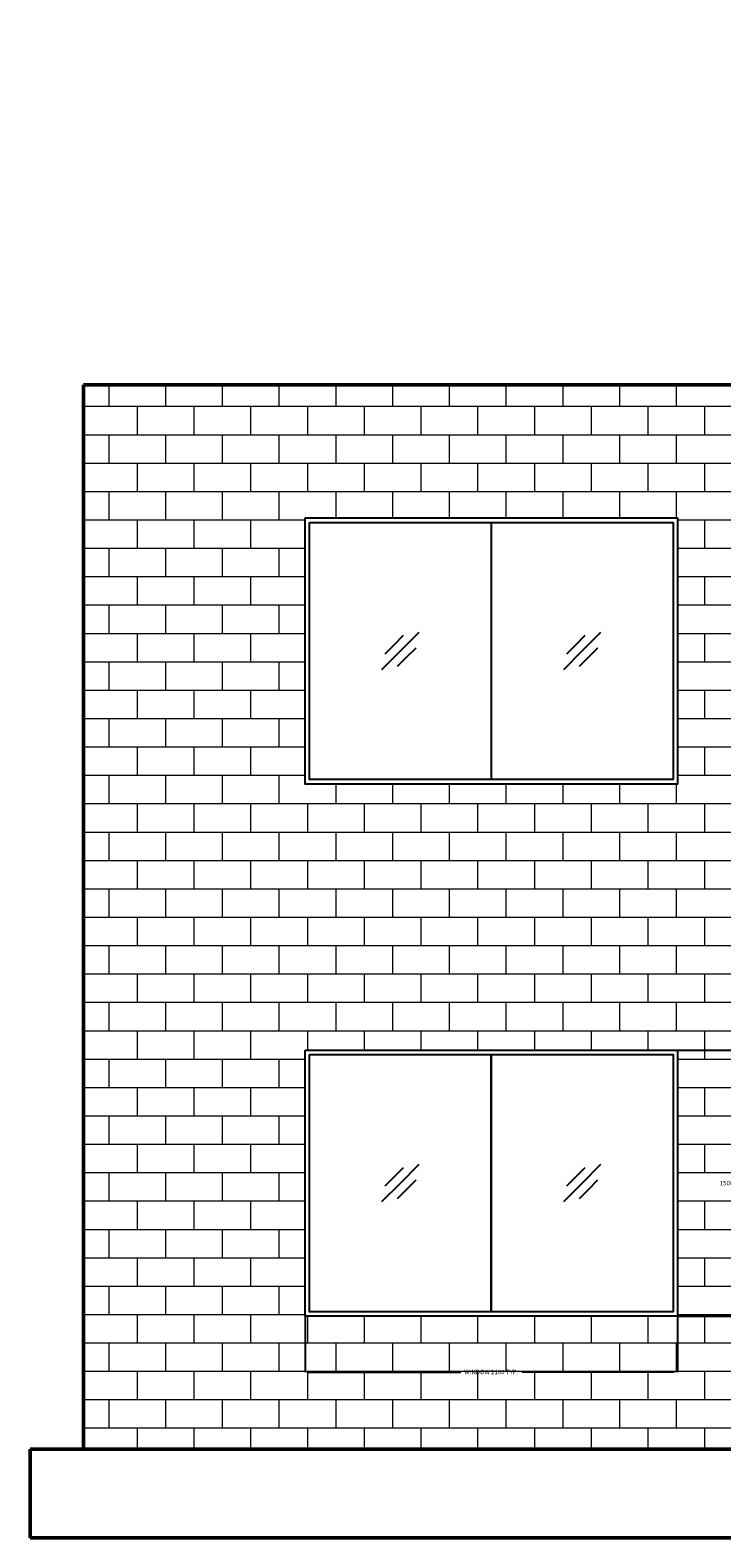
# Model space of a CAD drawing. Units: centimetres. Extents: x 2755 to 12755, y 4821 to 13321.
# Tile 1 of 2: x 2755 to 6655, y 4821 to 13321. Entities that reach past the tile are written whole.
import ezdxf

# ---------------------------------------------------------------- set-up
doc = ezdxf.new("R2010")
doc.units = ezdxf.units.CM
doc.header["$MEASUREMENT"] = 0
for name, color, linetype, lineweight in [('A-ANNO-DIMS', 2, 'Continuous', 18), ('A-GLAZ', 4, 'Continuous', 25), ('A-WALL', 7, 'Continuous', 50), ('A-WALL-PATT', 8, 'Continuous', 13)]:
    doc.layers.add(name, color=color, linetype=linetype, lineweight=lineweight)
doc.styles.get("Standard").update_dxf_attribs({"font": 'arial.ttf'})
doc.dimstyles.get("Standard").update_dxf_attribs({"dimtxt": 25, "dimasz": 20, "dimexe": 0.18, "dimexo": 0.0625, "dimgap": 10, "dimtad": 0, "dimtih": 1, "dimtoh": 1, "dimdec": 0, "dimzin": 0, "dimdsep": 46, "dimtxsty": 'Standard', "dimcen": 10, "dimadec": 0, "dimazin": 0, "dimtfac": 1, "dimtdec": 0, "dimtofl": 0, "dimtmove": 0, "dimatfit": 3, "dimfxl": 1, "dimtolj": 1, "dimtzin": 0, "dimarcsym": 0})

# ---------------------------------------------------------------- blocks, each defined once
blk = doc.blocks.new('WIN-2100')
blk.add_line((5355.3, 7545.8), (5355.3, 6095.8))
for points in [[(4305.3, 7570.8), (6405.3, 7570.8), (6405.3, 6070.8), (4305.3, 6070.8)], [(4330.3, 7545.8), (6380.3, 7545.8), (6380.3, 6095.8), (4330.3, 6095.8)]]:
    blk.add_lwpolyline(points, close=True)
blk = doc.blocks.new('*D4')
at = {"layer": 'A-ANNO-DIMS', "color": 0, "lineweight": -2, "transparency": 16777216}
for p, q in [((4305.3, 6070.8), (4305.3, 5755.6)), ((6405.3, 6070.8), (6405.3, 5755.6)), ((4325.3, 5755.8), (5183.1, 5755.8)), ((6385.3, 5755.8), (5527.6, 5755.8))]:
    blk.add_line(p, q, dxfattribs=at)
at = {"layer": 'A-ANNO-DIMS', "color": 0, "transparency": 16777216}
for points in [[(4325.3, 5759.2), (4325.3, 5752.5), (4305.3, 5755.8)], [(6385.3, 5759.2), (6385.3, 5752.5), (6405.3, 5755.8)]]:
    blk.add_solid(points, dxfattribs=at)
at = {"layer": 'Defpoints', "color": 0, "transparency": 16777216}
for p in [(4305.3, 6070.8), (6405.3, 6070.8), (6405.3, 5755.8)]:
    blk.add_point(p, dxfattribs=at)
at = {"layer": 'A-ANNO-DIMS', "color": 0, "transparency": 16777216, "insert": (5355.3, 5755.8), "char_height": 25, "attachment_point": 5}
blk.add_mtext('\\A1;WINDOW 2100 TYP.', dxfattribs=at)
blk = doc.blocks.new('*D5')
at = {"layer": 'A-ANNO-DIMS', "color": 0, "lineweight": -2, "transparency": 16777216}
for p, q in [((6405.4, 7570.8), (6720.5, 7570.8)), ((6720.3, 7550.8), (6720.3, 6843.6)), ((6720.3, 6090.8), (6720.3, 6798.1)), ((6405.4, 6070.8), (6720.5, 6070.8))]:
    blk.add_line(p, q, dxfattribs=at)
at = {"layer": 'A-ANNO-DIMS', "color": 0, "transparency": 16777216}
for points in [[(6717, 7550.8), (6723.7, 7550.8), (6720.3, 7570.8)], [(6717, 6090.8), (6723.7, 6090.8), (6720.3, 6070.8)]]:
    blk.add_solid(points, dxfattribs=at)
at = {"layer": 'Defpoints', "color": 0, "transparency": 16777216}
for p in [(6405.3, 7570.8), (6720.3, 7570.8), (6405.3, 6070.8)]:
    blk.add_point(p, dxfattribs=at)
at = {"layer": 'A-ANNO-DIMS', "color": 0, "transparency": 16777216, "insert": (6720.3, 6820.8), "char_height": 25, "attachment_point": 5}
blk.add_mtext('\\A1;1500 TYP.', dxfattribs=at)

msp = doc.modelspace()

# ---------------------------------------------------------------- hatches: boundary and pattern name
at = {"layer": 'A-WALL-PATT'}
h = msp.add_hatch(dxfattribs=at)
h.set_pattern_fill('AR-B816', color=256, scale=20)
h.paths.add_polyline_path([(7655.3, 11320.8), (3055.3, 11320.8), (3055.3, 5320.8), (7655.3, 5320.8)])
h.paths.add_polyline_path([(4305.3, 7570.8), (6405.3, 7570.8), (6405.3, 6070.8), (4305.3, 6070.8)], flags=16)
h.paths.add_polyline_path([(4330.3, 7545.8), (6380.3, 7545.8), (6380.3, 6095.8), (4330.3, 6095.8)], flags=0)
h.paths.add_polyline_path([(4305.3, 9070.8), (4305.3, 10570.8), (6405.3, 10570.8), (6405.3, 9070.8)], flags=16)
h.paths.add_polyline_path([(4330.3, 9095.8), (4330.3, 10545.8), (6380.3, 10545.8), (6380.3, 9095.8)], flags=0)
h.paths.add_polyline_path([(9955.3, 12820.8), (11955.3, 12820.8), (11955.3, 5320.8), (12455.3, 5320.8), (12455.3, 13320.8), (9455.3, 13320.8), (9455.3, 11320.8), (9455.3, 5320.8), (9955.3, 5320.8)])

# ---------------------------------------------------------------- linework, layer by layer
at = {"layer": 'A-GLAZ'}
for p, q in [((4807.5, 9856.2), (4860.5, 9909.2)), ((4842.8, 9820.8), (4948.9, 9926.9)), ((5832.5, 9856.2), (5885.5, 9909.2)), ((5867.8, 9820.8), (5973.9, 9926.9)), ((4842.8, 9820.8), (4736.8, 9714.8)), ((4807.5, 9856.2), (4754.4, 9803.1)), ((4878.2, 9785.5), (4825.1, 9732.4)), ((4878.2, 9785.5), (4931.2, 9838.5)), ((5867.8, 9820.8), (5761.8, 9714.8)), ((5832.5, 9856.2), (5779.4, 9803.1)), ((5903.2, 9785.5), (5850.1, 9732.4)), ((5903.2, 9785.5), (5956.2, 9838.5)), ((5355.3, 6095.8), (5355.3, 7545.8)), ((4807.5, 6856.2), (4860.5, 6909.2)), ((4842.8, 6820.8), (4948.9, 6926.9)), ((5832.5, 6856.2), (5885.5, 6909.2)), ((5867.8, 6820.8), (5973.9, 6926.9)), ((4842.8, 6820.8), (4736.8, 6714.8)), ((4807.5, 6856.2), (4754.4, 6803.1)), ((4878.2, 6785.5), (4931.2, 6838.5)), ((5867.8, 6820.8), (5761.8, 6714.8)), ((5832.5, 6856.2), (5779.4, 6803.1)), ((5903.2, 6785.5), (5956.2, 6838.5)), ((4878.2, 6785.5), (4825.1, 6732.4)), ((5903.2, 6785.5), (5850.1, 6732.4))]:
    msp.add_line(p, q, dxfattribs=at)
at = {"layer": 'A-WALL'}
for p, q in [((9455.3, 11320.8), (3055.3, 11320.8)), ((3055.3, 5320.8), (3055.3, 11320.8)), ((12755.3, 5320.8), (2755.3, 5320.8)), ((2755.3, 5320.8), (3055.3, 5320.8)), ((2755.3, 5320.8), (2755.3, 4820.8)), ((2755.3, 4820.8), (12755.3, 4820.8))]:
    msp.add_line(p, q, dxfattribs=at)

# ---------------------------------------------------------------- block references
at = {"layer": 'A-GLAZ'}
for p in [(0, 3000), (0, 0)]:
    msp.add_blockref('WIN-2100', p, dxfattribs=at)

# ---------------------------------------------------------------- dimensions: what is measured, and where the dimension line sits
at = {"layer": 'A-ANNO-DIMS'}
dim = msp.add_linear_dim(base=(6720.3, 7570.8), p1=(6405.3, 6070.8), p2=(6405.3, 7570.8), angle=90, text='<> TYP.', dimstyle='Standard', override={"dimdec": 0, "dimlfac": 1, "dimrnd": 0, "dimzin": 0, "dimdsep": 46, "dimlunit": 2}, dxfattribs=at)
dim.commit()
dim.dimension.update_dxf_attribs({"geometry": '*D5', "text_midpoint": (6720.3, 6820.8)})
dim = msp.add_linear_dim(base=(6405.3, 5755.8), p1=(4305.3, 6070.8), p2=(6405.3, 6070.8), text='WINDOW <> TYP.', dimstyle='Standard', override={"dimdec": 0, "dimlfac": 1, "dimrnd": 0, "dimzin": 0, "dimdsep": 46, "dimlunit": 2}, dxfattribs=at)
dim.commit()
dim.dimension.update_dxf_attribs({"geometry": '*D4', "text_midpoint": (5355.3, 5755.8)})

doc.saveas('drawing.dxf')
